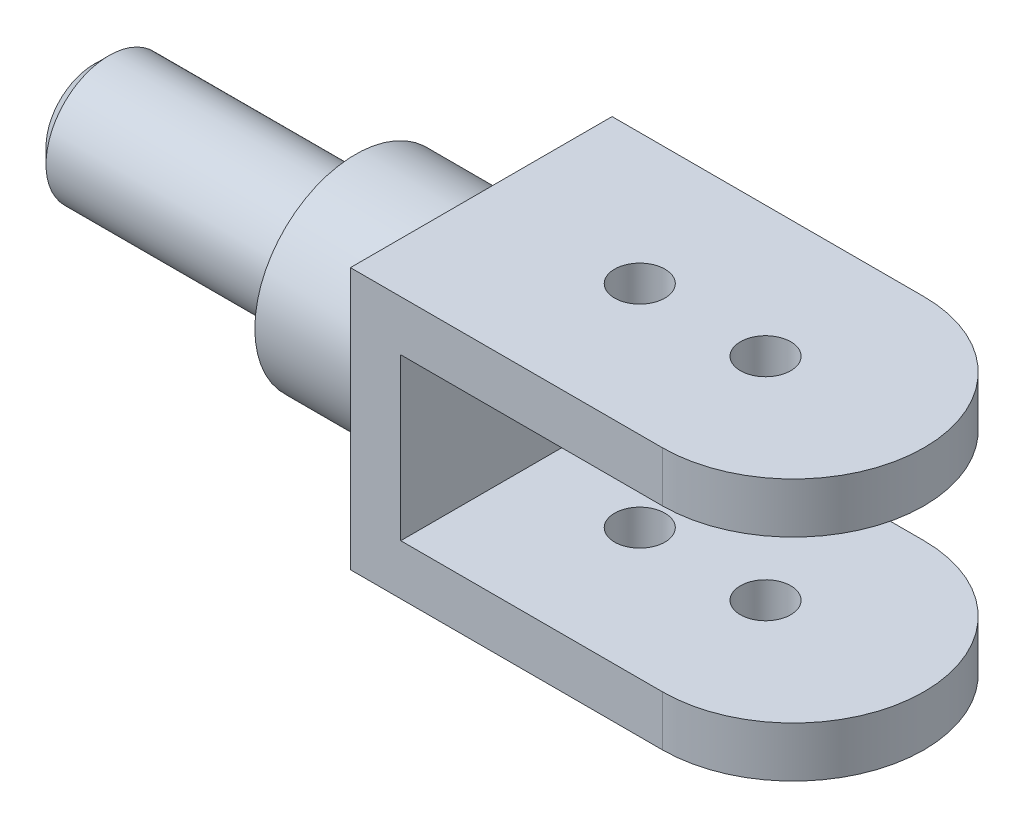
ISO-10303-21;
HEADER;
FILE_DESCRIPTION(('STEP AP214'),'2;1');
FILE_NAME('part.step','',(''),(''),'','','');
FILE_SCHEMA(('AUTOMOTIVE_DESIGN { 1 0 10303 214 1 1 1 1 }'));
ENDSEC;
DATA;
#1=APPLICATION_CONTEXT('core data for automotive mechanical design processes');
#2=APPLICATION_PROTOCOL_DEFINITION('international standard','automotive_design',2000,#1);
#3=PRODUCT_CONTEXT('',#1,'mechanical');
#4=PRODUCT('Part','Part','',(#3));
#5=PRODUCT_RELATED_PRODUCT_CATEGORY('part','',(#4));
#6=PRODUCT_DEFINITION_FORMATION('','',#4);
#7=PRODUCT_DEFINITION_CONTEXT('part definition',#1,'design');
#8=PRODUCT_DEFINITION('design','',#6,#7);
#9=PRODUCT_DEFINITION_SHAPE('','',#8);
#10=(LENGTH_UNIT() NAMED_UNIT(*) SI_UNIT(.MILLI.,.METRE.));
#11=(NAMED_UNIT(*) PLANE_ANGLE_UNIT() SI_UNIT($,.RADIAN.));
#12=(NAMED_UNIT(*) SI_UNIT($,.STERADIAN.) SOLID_ANGLE_UNIT());
#13=UNCERTAINTY_MEASURE_WITH_UNIT(LENGTH_MEASURE(1.E-05),#10,'distance_accuracy_value','');
#14=(GEOMETRIC_REPRESENTATION_CONTEXT(3) GLOBAL_UNCERTAINTY_ASSIGNED_CONTEXT((#13)) GLOBAL_UNIT_ASSIGNED_CONTEXT((#10,
#11,#12)) REPRESENTATION_CONTEXT('',''));
#15=CARTESIAN_POINT('',(0.,0.,0.));
#16=DIRECTION('',(0.,0.,1.));
#17=DIRECTION('',(1.,0.,0.));
#18=AXIS2_PLACEMENT_3D('',#15,#16,#17);
#19=CARTESIAN_POINT('',(0.,-52.,52.));
#20=DIRECTION('',(1.,0.,0.));
#21=DIRECTION('',(0.,0.,-1.));
#22=AXIS2_PLACEMENT_3D('',#19,#20,#21);
#23=PLANE('',#22);
#24=CARTESIAN_POINT('',(0.,-26.,26.));
#25=DIRECTION('',(1.,0.,0.));
#26=DIRECTION('',(0.,0.,-1.));
#27=AXIS2_PLACEMENT_3D('',#24,#25,#26);
#28=CIRCLE('',#27,23.);
#29=CARTESIAN_POINT('',(0.,-26.,3.00000000000002));
#30=VERTEX_POINT('',#29);
#31=EDGE_CURVE('E164',#30,#30,#28,.T.);
#32=ORIENTED_EDGE('',*,*,#31,.T.);
#33=EDGE_LOOP('',(#32));
#34=FACE_BOUND('',#33,.T.);
#35=DIRECTION('',(0.,-1.,0.));
#36=VECTOR('',#35,1.);
#37=CARTESIAN_POINT('',(0.,-52.,0.));
#38=LINE('',#37,#36);
#39=CARTESIAN_POINT('',(0.,0.,0.));
#40=VERTEX_POINT('',#39);
#41=CARTESIAN_POINT('',(0.,-52.,0.));
#42=VERTEX_POINT('',#41);
#43=EDGE_CURVE('E141',#40,#42,#38,.T.);
#44=ORIENTED_EDGE('',*,*,#43,.T.);
#45=DIRECTION('',(0.,0.,-1.));
#46=VECTOR('',#45,1.);
#47=CARTESIAN_POINT('',(0.,-52.,52.));
#48=LINE('',#47,#46);
#49=CARTESIAN_POINT('',(0.,-52.,52.));
#50=VERTEX_POINT('',#49);
#51=EDGE_CURVE('E159',#50,#42,#48,.T.);
#52=ORIENTED_EDGE('',*,*,#51,.F.);
#53=DIRECTION('',(0.,-1.,0.));
#54=VECTOR('',#53,1.);
#55=CARTESIAN_POINT('',(0.,-52.,52.));
#56=LINE('',#55,#54);
#57=CARTESIAN_POINT('',(0.,0.,52.));
#58=VERTEX_POINT('',#57);
#59=EDGE_CURVE('E146',#58,#50,#56,.T.);
#60=ORIENTED_EDGE('',*,*,#59,.F.);
#61=DIRECTION('',(0.,0.,-1.));
#62=VECTOR('',#61,1.);
#63=CARTESIAN_POINT('',(0.,0.,52.));
#64=LINE('',#63,#62);
#65=EDGE_CURVE('E153',#58,#40,#64,.T.);
#66=ORIENTED_EDGE('',*,*,#65,.T.);
#67=EDGE_LOOP('',(#44,#52,#60,#66));
#68=FACE_BOUND('',#67,.T.);
#69=ADVANCED_FACE('F50',(#34,#68),#23,.F.);
#70=CARTESIAN_POINT('',(88.,-52.,52.));
#71=DIRECTION('',(0.,1.,0.));
#72=DIRECTION('',(0.,0.,1.));
#73=AXIS2_PLACEMENT_3D('',#70,#71,#72);
#74=PLANE('',#73);
#75=CARTESIAN_POINT('',(31.5,-52.,26.));
#76=DIRECTION('',(0.,-1.,0.));
#77=DIRECTION('',(0.,0.,-1.));
#78=AXIS2_PLACEMENT_3D('',#75,#76,#77);
#79=CIRCLE('',#78,5.);
#80=CARTESIAN_POINT('',(31.5,-52.,21.));
#81=VERTEX_POINT('',#80);
#82=EDGE_CURVE('E512',#81,#81,#79,.T.);
#83=ORIENTED_EDGE('',*,*,#82,.F.);
#84=EDGE_LOOP('',(#83));
#85=FACE_BOUND('',#84,.T.);
#86=CARTESIAN_POINT('',(56.5,-52.,26.));
#87=DIRECTION('',(0.,-1.,0.));
#88=DIRECTION('',(0.,0.,-1.));
#89=AXIS2_PLACEMENT_3D('',#86,#87,#88);
#90=CIRCLE('',#89,5.);
#91=CARTESIAN_POINT('',(56.5,-52.,21.));
#92=VERTEX_POINT('',#91);
#93=EDGE_CURVE('E504',#92,#92,#90,.T.);
#94=ORIENTED_EDGE('',*,*,#93,.F.);
#95=EDGE_LOOP('',(#94));
#96=FACE_BOUND('',#95,.T.);
#97=DIRECTION('',(1.,0.,0.));
#98=VECTOR('',#97,1.);
#99=CARTESIAN_POINT('',(88.,-52.,0.));
#100=LINE('',#99,#98);
#101=CARTESIAN_POINT('',(62.,-52.,0.));
#102=VERTEX_POINT('',#101);
#103=EDGE_CURVE('E201',#42,#102,#100,.T.);
#104=ORIENTED_EDGE('',*,*,#103,.T.);
#105=CARTESIAN_POINT('',(62.,-52.,26.));
#106=DIRECTION('',(0.,-1.,0.));
#107=DIRECTION('',(0.,0.,-1.));
#108=AXIS2_PLACEMENT_3D('',#105,#106,#107);
#109=CIRCLE('',#108,26.);
#110=CARTESIAN_POINT('',(62.,-52.,52.));
#111=VERTEX_POINT('',#110);
#112=EDGE_CURVE('E131',#102,#111,#109,.T.);
#113=ORIENTED_EDGE('',*,*,#112,.T.);
#114=DIRECTION('',(1.,0.,0.));
#115=VECTOR('',#114,1.);
#116=CARTESIAN_POINT('',(88.,-52.,52.));
#117=LINE('',#116,#115);
#118=EDGE_CURVE('E100',#50,#111,#117,.T.);
#119=ORIENTED_EDGE('',*,*,#118,.F.);
#120=ORIENTED_EDGE('',*,*,#51,.T.);
#121=EDGE_LOOP('',(#104,#113,#119,#120));
#122=FACE_BOUND('',#121,.T.);
#123=ADVANCED_FACE('F213',(#85,#96,#122),#74,.F.);
#124=CARTESIAN_POINT('',(9.99999999999999,-42.,52.));
#125=DIRECTION('',(0.,-1.,0.));
#126=DIRECTION('',(0.,0.,-1.));
#127=AXIS2_PLACEMENT_3D('',#124,#125,#126);
#128=PLANE('',#127);
#129=CARTESIAN_POINT('',(31.5,-42.,26.));
#130=DIRECTION('',(0.,-1.,0.));
#131=DIRECTION('',(0.,0.,-1.));
#132=AXIS2_PLACEMENT_3D('',#129,#130,#131);
#133=CIRCLE('',#132,5.);
#134=CARTESIAN_POINT('',(31.5,-42.,21.));
#135=VERTEX_POINT('',#134);
#136=EDGE_CURVE('E180',#135,#135,#133,.T.);
#137=ORIENTED_EDGE('',*,*,#136,.T.);
#138=EDGE_LOOP('',(#137));
#139=FACE_BOUND('',#138,.T.);
#140=CARTESIAN_POINT('',(56.5,-42.,26.));
#141=DIRECTION('',(0.,-1.,0.));
#142=DIRECTION('',(0.,0.,-1.));
#143=AXIS2_PLACEMENT_3D('',#140,#141,#142);
#144=CIRCLE('',#143,5.);
#145=CARTESIAN_POINT('',(56.5,-42.,21.));
#146=VERTEX_POINT('',#145);
#147=EDGE_CURVE('E492',#146,#146,#144,.T.);
#148=ORIENTED_EDGE('',*,*,#147,.T.);
#149=EDGE_LOOP('',(#148));
#150=FACE_BOUND('',#149,.T.);
#151=DIRECTION('',(-1.,0.,0.));
#152=VECTOR('',#151,1.);
#153=CARTESIAN_POINT('',(9.99999999999999,-42.,52.));
#154=LINE('',#153,#152);
#155=CARTESIAN_POINT('',(62.,-42.,52.));
#156=VERTEX_POINT('',#155);
#157=CARTESIAN_POINT('',(9.99999999999999,-42.,52.));
#158=VERTEX_POINT('',#157);
#159=EDGE_CURVE('E195',#156,#158,#154,.T.);
#160=ORIENTED_EDGE('',*,*,#159,.F.);
#161=CARTESIAN_POINT('',(62.,-42.,26.));
#162=DIRECTION('',(0.,-1.,0.));
#163=DIRECTION('',(0.,0.,-1.));
#164=AXIS2_PLACEMENT_3D('',#161,#162,#163);
#165=CIRCLE('',#164,26.);
#166=CARTESIAN_POINT('',(62.,-42.,0.));
#167=VERTEX_POINT('',#166);
#168=EDGE_CURVE('E182',#167,#156,#165,.T.);
#169=ORIENTED_EDGE('',*,*,#168,.F.);
#170=DIRECTION('',(-1.,0.,0.));
#171=VECTOR('',#170,1.);
#172=CARTESIAN_POINT('',(9.99999999999999,-42.,0.));
#173=LINE('',#172,#171);
#174=CARTESIAN_POINT('',(9.99999999999999,-42.,0.));
#175=VERTEX_POINT('',#174);
#176=EDGE_CURVE('E152',#167,#175,#173,.T.);
#177=ORIENTED_EDGE('',*,*,#176,.T.);
#178=DIRECTION('',(0.,0.,-1.));
#179=VECTOR('',#178,1.);
#180=CARTESIAN_POINT('',(9.99999999999999,-42.,52.));
#181=LINE('',#180,#179);
#182=EDGE_CURVE('E157',#158,#175,#181,.T.);
#183=ORIENTED_EDGE('',*,*,#182,.F.);
#184=EDGE_LOOP('',(#160,#169,#177,#183));
#185=FACE_BOUND('',#184,.T.);
#186=ADVANCED_FACE('F207',(#139,#150,#185),#128,.F.);
#187=CARTESIAN_POINT('',(9.99999999999999,-10.,52.));
#188=DIRECTION('',(-1.,0.,0.));
#189=DIRECTION('',(0.,0.,1.));
#190=AXIS2_PLACEMENT_3D('',#187,#188,#189);
#191=PLANE('',#190);
#192=DIRECTION('',(0.,1.,0.));
#193=VECTOR('',#192,1.);
#194=CARTESIAN_POINT('',(9.99999999999999,-10.,0.));
#195=LINE('',#194,#193);
#196=CARTESIAN_POINT('',(9.99999999999999,-10.,0.));
#197=VERTEX_POINT('',#196);
#198=EDGE_CURVE('E81',#175,#197,#195,.T.);
#199=ORIENTED_EDGE('',*,*,#198,.T.);
#200=DIRECTION('',(0.,0.,-1.));
#201=VECTOR('',#200,1.);
#202=CARTESIAN_POINT('',(9.99999999999999,-10.,52.));
#203=LINE('',#202,#201);
#204=CARTESIAN_POINT('',(9.99999999999999,-10.,52.));
#205=VERTEX_POINT('',#204);
#206=EDGE_CURVE('E150',#205,#197,#203,.T.);
#207=ORIENTED_EDGE('',*,*,#206,.F.);
#208=DIRECTION('',(0.,1.,0.));
#209=VECTOR('',#208,1.);
#210=CARTESIAN_POINT('',(9.99999999999999,-10.,52.));
#211=LINE('',#210,#209);
#212=EDGE_CURVE('E191',#158,#205,#211,.T.);
#213=ORIENTED_EDGE('',*,*,#212,.F.);
#214=ORIENTED_EDGE('',*,*,#182,.T.);
#215=EDGE_LOOP('',(#199,#207,#213,#214));
#216=FACE_BOUND('',#215,.T.);
#217=ADVANCED_FACE('F209',(#216),#191,.F.);
#218=CARTESIAN_POINT('',(88.,-10.,52.));
#219=DIRECTION('',(0.,1.,0.));
#220=DIRECTION('',(0.,0.,1.));
#221=AXIS2_PLACEMENT_3D('',#218,#219,#220);
#222=PLANE('',#221);
#223=CARTESIAN_POINT('',(31.5,-10.,26.));
#224=DIRECTION('',(0.,1.,0.));
#225=DIRECTION('',(0.,0.,1.));
#226=AXIS2_PLACEMENT_3D('',#223,#224,#225);
#227=CIRCLE('',#226,5.);
#228=CARTESIAN_POINT('',(31.5,-10.,21.));
#229=VERTEX_POINT('',#228);
#230=EDGE_CURVE('E500',#229,#229,#227,.T.);
#231=ORIENTED_EDGE('',*,*,#230,.T.);
#232=EDGE_LOOP('',(#231));
#233=FACE_BOUND('',#232,.T.);
#234=CARTESIAN_POINT('',(56.5,-10.,26.));
#235=DIRECTION('',(0.,1.,0.));
#236=DIRECTION('',(0.,0.,1.));
#237=AXIS2_PLACEMENT_3D('',#234,#235,#236);
#238=CIRCLE('',#237,5.);
#239=CARTESIAN_POINT('',(56.5,-10.,21.));
#240=VERTEX_POINT('',#239);
#241=EDGE_CURVE('E498',#240,#240,#238,.T.);
#242=ORIENTED_EDGE('',*,*,#241,.T.);
#243=EDGE_LOOP('',(#242));
#244=FACE_BOUND('',#243,.T.);
#245=DIRECTION('',(1.,0.,0.));
#246=VECTOR('',#245,1.);
#247=CARTESIAN_POINT('',(88.,-10.,0.));
#248=LINE('',#247,#246);
#249=CARTESIAN_POINT('',(62.,-10.,0.));
#250=VERTEX_POINT('',#249);
#251=EDGE_CURVE('E142',#197,#250,#248,.T.);
#252=ORIENTED_EDGE('',*,*,#251,.T.);
#253=CARTESIAN_POINT('',(62.,-10.,26.));
#254=DIRECTION('',(0.,1.,0.));
#255=DIRECTION('',(0.,0.,1.));
#256=AXIS2_PLACEMENT_3D('',#253,#254,#255);
#257=CIRCLE('',#256,26.);
#258=CARTESIAN_POINT('',(62.,-10.,52.));
#259=VERTEX_POINT('',#258);
#260=EDGE_CURVE('E123',#259,#250,#257,.T.);
#261=ORIENTED_EDGE('',*,*,#260,.F.);
#262=DIRECTION('',(1.,0.,0.));
#263=VECTOR('',#262,1.);
#264=CARTESIAN_POINT('',(88.,-10.,52.));
#265=LINE('',#264,#263);
#266=EDGE_CURVE('E197',#205,#259,#265,.T.);
#267=ORIENTED_EDGE('',*,*,#266,.F.);
#268=ORIENTED_EDGE('',*,*,#206,.T.);
#269=EDGE_LOOP('',(#252,#261,#267,#268));
#270=FACE_BOUND('',#269,.T.);
#271=ADVANCED_FACE('F147',(#233,#244,#270),#222,.F.);
#272=CARTESIAN_POINT('',(0.,0.,52.));
#273=DIRECTION('',(0.,-1.,0.));
#274=DIRECTION('',(0.,0.,-1.));
#275=AXIS2_PLACEMENT_3D('',#272,#273,#274);
#276=PLANE('',#275);
#277=CARTESIAN_POINT('',(31.5,0.,26.));
#278=DIRECTION('',(0.,-1.,0.));
#279=DIRECTION('',(0.,0.,-1.));
#280=AXIS2_PLACEMENT_3D('',#277,#278,#279);
#281=CIRCLE('',#280,5.);
#282=CARTESIAN_POINT('',(31.5,0.,21.));
#283=VERTEX_POINT('',#282);
#284=EDGE_CURVE('E505',#283,#283,#281,.T.);
#285=ORIENTED_EDGE('',*,*,#284,.T.);
#286=EDGE_LOOP('',(#285));
#287=FACE_BOUND('',#286,.T.);
#288=CARTESIAN_POINT('',(56.5,0.,26.));
#289=DIRECTION('',(0.,-1.,0.));
#290=DIRECTION('',(0.,0.,-1.));
#291=AXIS2_PLACEMENT_3D('',#288,#289,#290);
#292=CIRCLE('',#291,5.);
#293=CARTESIAN_POINT('',(56.5,0.,21.));
#294=VERTEX_POINT('',#293);
#295=EDGE_CURVE('E507',#294,#294,#292,.T.);
#296=ORIENTED_EDGE('',*,*,#295,.T.);
#297=EDGE_LOOP('',(#296));
#298=FACE_BOUND('',#297,.T.);
#299=DIRECTION('',(-1.,0.,0.));
#300=VECTOR('',#299,1.);
#301=CARTESIAN_POINT('',(0.,0.,52.));
#302=LINE('',#301,#300);
#303=CARTESIAN_POINT('',(62.,0.,52.));
#304=VERTEX_POINT('',#303);
#305=EDGE_CURVE('E63',#304,#58,#302,.T.);
#306=ORIENTED_EDGE('',*,*,#305,.F.);
#307=CARTESIAN_POINT('',(62.,0.,26.));
#308=DIRECTION('',(0.,1.,0.));
#309=DIRECTION('',(0.,0.,1.));
#310=AXIS2_PLACEMENT_3D('',#307,#308,#309);
#311=CIRCLE('',#310,26.);
#312=CARTESIAN_POINT('',(62.,0.,0.));
#313=VERTEX_POINT('',#312);
#314=EDGE_CURVE('E133',#304,#313,#311,.T.);
#315=ORIENTED_EDGE('',*,*,#314,.T.);
#316=DIRECTION('',(-1.,0.,0.));
#317=VECTOR('',#316,1.);
#318=CARTESIAN_POINT('',(0.,0.,0.));
#319=LINE('',#318,#317);
#320=EDGE_CURVE('E91',#313,#40,#319,.T.);
#321=ORIENTED_EDGE('',*,*,#320,.T.);
#322=ORIENTED_EDGE('',*,*,#65,.F.);
#323=EDGE_LOOP('',(#306,#315,#321,#322));
#324=FACE_BOUND('',#323,.T.);
#325=ADVANCED_FACE('F220',(#287,#298,#324),#276,.F.);
#326=CARTESIAN_POINT('',(0.,0.,52.));
#327=DIRECTION('',(0.,0.,-1.));
#328=DIRECTION('',(-1.,0.,0.));
#329=AXIS2_PLACEMENT_3D('',#326,#327,#328);
#330=PLANE('',#329);
#331=ORIENTED_EDGE('',*,*,#118,.T.);
#332=DIRECTION('',(0.,-1.,0.));
#333=VECTOR('',#332,1.);
#334=CARTESIAN_POINT('',(62.,18.,52.));
#335=LINE('',#334,#333);
#336=EDGE_CURVE('E187',#156,#111,#335,.T.);
#337=ORIENTED_EDGE('',*,*,#336,.F.);
#338=ORIENTED_EDGE('',*,*,#159,.T.);
#339=ORIENTED_EDGE('',*,*,#212,.T.);
#340=ORIENTED_EDGE('',*,*,#266,.T.);
#341=EDGE_CURVE('E126',#304,#259,#335,.T.);
#342=ORIENTED_EDGE('',*,*,#341,.F.);
#343=ORIENTED_EDGE('',*,*,#305,.T.);
#344=ORIENTED_EDGE('',*,*,#59,.T.);
#345=EDGE_LOOP('',(#331,#337,#338,#339,#340,#342,#343,#344));
#346=FACE_BOUND('',#345,.T.);
#347=ADVANCED_FACE('F208',(#346),#330,.F.);
#348=CARTESIAN_POINT('',(0.,0.,0.));
#349=DIRECTION('',(0.,0.,-1.));
#350=DIRECTION('',(-1.,0.,0.));
#351=AXIS2_PLACEMENT_3D('',#348,#349,#350);
#352=PLANE('',#351);
#353=DIRECTION('',(0.,-1.,0.));
#354=VECTOR('',#353,1.);
#355=CARTESIAN_POINT('',(62.,18.,0.));
#356=LINE('',#355,#354);
#357=EDGE_CURVE('E144',#167,#102,#356,.T.);
#358=ORIENTED_EDGE('',*,*,#357,.T.);
#359=ORIENTED_EDGE('',*,*,#103,.F.);
#360=ORIENTED_EDGE('',*,*,#43,.F.);
#361=ORIENTED_EDGE('',*,*,#320,.F.);
#362=EDGE_CURVE('E129',#313,#250,#356,.T.);
#363=ORIENTED_EDGE('',*,*,#362,.T.);
#364=ORIENTED_EDGE('',*,*,#251,.F.);
#365=ORIENTED_EDGE('',*,*,#198,.F.);
#366=ORIENTED_EDGE('',*,*,#176,.F.);
#367=EDGE_LOOP('',(#358,#359,#360,#361,#363,#364,#365,#366));
#368=FACE_BOUND('',#367,.T.);
#369=ADVANCED_FACE('F139',(#368),#352,.T.);
#370=CARTESIAN_POINT('',(62.,-42.,26.));
#371=DIRECTION('',(0.,-1.,0.));
#372=DIRECTION('',(0.,0.,-1.));
#373=AXIS2_PLACEMENT_3D('',#370,#371,#372);
#374=CYLINDRICAL_SURFACE('',#373,26.);
#375=ORIENTED_EDGE('',*,*,#112,.F.);
#376=ORIENTED_EDGE('',*,*,#357,.F.);
#377=ORIENTED_EDGE('',*,*,#168,.T.);
#378=ORIENTED_EDGE('',*,*,#336,.T.);
#379=EDGE_LOOP('',(#375,#376,#377,#378));
#380=FACE_BOUND('',#379,.T.);
#381=ADVANCED_FACE('F214',(#380),#374,.T.);
#382=CARTESIAN_POINT('',(62.,-10.,26.));
#383=DIRECTION('',(0.,1.,0.));
#384=DIRECTION('',(0.,0.,1.));
#385=AXIS2_PLACEMENT_3D('',#382,#383,#384);
#386=CYLINDRICAL_SURFACE('',#385,26.);
#387=ORIENTED_EDGE('',*,*,#314,.F.);
#388=ORIENTED_EDGE('',*,*,#341,.T.);
#389=ORIENTED_EDGE('',*,*,#260,.T.);
#390=ORIENTED_EDGE('',*,*,#362,.F.);
#391=EDGE_LOOP('',(#387,#388,#389,#390));
#392=FACE_BOUND('',#391,.T.);
#393=ADVANCED_FACE('F130',(#392),#386,.T.);
#394=CARTESIAN_POINT('',(-25.,-26.,26.));
#395=DIRECTION('',(1.,0.,0.));
#396=DIRECTION('',(0.,0.,-1.));
#397=AXIS2_PLACEMENT_3D('',#394,#395,#396);
#398=CYLINDRICAL_SURFACE('',#397,20.);
#399=CARTESIAN_POINT('',(-3.00000000000002,-26.,26.));
#400=DIRECTION('',(1.,0.,0.));
#401=DIRECTION('',(0.,0.,-1.));
#402=AXIS2_PLACEMENT_3D('',#399,#400,#401);
#403=CIRCLE('',#402,20.);
#404=CARTESIAN_POINT('',(-3.00000000000002,-26.,6.));
#405=VERTEX_POINT('',#404);
#406=EDGE_CURVE('E162',#405,#405,#403,.F.);
#407=ORIENTED_EDGE('',*,*,#406,.T.);
#408=EDGE_LOOP('',(#407));
#409=FACE_BOUND('',#408,.T.);
#410=CARTESIAN_POINT('',(-25.,-26.,26.));
#411=DIRECTION('',(-1.,0.,0.));
#412=DIRECTION('',(0.,0.,1.));
#413=AXIS2_PLACEMENT_3D('',#410,#411,#412);
#414=CIRCLE('',#413,20.);
#415=CARTESIAN_POINT('',(-25.,-26.,46.));
#416=VERTEX_POINT('',#415);
#417=EDGE_CURVE('E177',#416,#416,#414,.T.);
#418=ORIENTED_EDGE('',*,*,#417,.F.);
#419=EDGE_LOOP('',(#418));
#420=FACE_BOUND('',#419,.T.);
#421=ADVANCED_FACE('F258',(#409,#420),#398,.T.);
#422=CARTESIAN_POINT('',(-25.,-26.,26.));
#423=DIRECTION('',(-1.,0.,0.));
#424=DIRECTION('',(0.,0.,1.));
#425=AXIS2_PLACEMENT_3D('',#422,#423,#424);
#426=PLANE('',#425);
#427=CARTESIAN_POINT('',(-25.,-26.,26.));
#428=DIRECTION('',(-1.,0.,0.));
#429=DIRECTION('',(0.,0.,1.));
#430=AXIS2_PLACEMENT_3D('',#427,#428,#429);
#431=CIRCLE('',#430,12.5);
#432=CARTESIAN_POINT('',(-25.,-26.,13.5));
#433=VERTEX_POINT('',#432);
#434=EDGE_CURVE('E170',#433,#433,#431,.T.);
#435=ORIENTED_EDGE('',*,*,#434,.F.);
#436=EDGE_LOOP('',(#435));
#437=FACE_BOUND('',#436,.T.);
#438=ORIENTED_EDGE('',*,*,#417,.T.);
#439=EDGE_LOOP('',(#438));
#440=FACE_BOUND('',#439,.T.);
#441=ADVANCED_FACE('F249',(#437,#440),#426,.T.);
#442=CARTESIAN_POINT('',(-3.00000000000002,-26.,26.));
#443=DIRECTION('',(1.,0.,0.));
#444=DIRECTION('',(0.,0.,-1.));
#445=AXIS2_PLACEMENT_3D('',#442,#443,#444);
#446=CONICAL_SURFACE('',#445,20.,0.785398163397443);
#447=ORIENTED_EDGE('',*,*,#31,.F.);
#448=EDGE_LOOP('',(#447));
#449=FACE_BOUND('',#448,.T.);
#450=ORIENTED_EDGE('',*,*,#406,.F.);
#451=EDGE_LOOP('',(#450));
#452=FACE_BOUND('',#451,.T.);
#453=ADVANCED_FACE('F244',(#449,#452),#446,.T.);
#454=CARTESIAN_POINT('',(-77.,-26.,26.));
#455=DIRECTION('',(1.,0.,0.));
#456=DIRECTION('',(0.,0.,-1.));
#457=AXIS2_PLACEMENT_3D('',#454,#455,#456);
#458=CYLINDRICAL_SURFACE('',#457,12.5);
#459=CARTESIAN_POINT('',(-74.0000000000001,-26.,26.));
#460=DIRECTION('',(-1.,0.,0.));
#461=DIRECTION('',(0.,0.,1.));
#462=AXIS2_PLACEMENT_3D('',#459,#460,#461);
#463=CIRCLE('',#462,12.5);
#464=CARTESIAN_POINT('',(-74.0000000000001,-26.,13.5));
#465=VERTEX_POINT('',#464);
#466=EDGE_CURVE('E11',#465,#465,#463,.F.);
#467=CARTESIAN_POINT('',(-74.0000000000001,-26.,13.5));
#468=CARTESIAN_POINT('',(-73.4895833333334,-26.,13.5));
#469=CARTESIAN_POINT('',(-72.9791666666668,-26.,13.5));
#470=CARTESIAN_POINT('',(-71.9583333333334,-26.,13.5));
#471=CARTESIAN_POINT('',(-71.4479166666668,-26.,13.5));
#472=CARTESIAN_POINT('',(-70.4270833333334,-26.,13.5));
#473=CARTESIAN_POINT('',(-69.9166666666668,-26.,13.5));
#474=CARTESIAN_POINT('',(-68.8958333333334,-26.,13.5));
#475=CARTESIAN_POINT('',(-68.3854166666668,-26.,13.5));
#476=CARTESIAN_POINT('',(-67.3645833333334,-26.,13.5));
#477=CARTESIAN_POINT('',(-66.8541666666668,-26.,13.5));
#478=CARTESIAN_POINT('',(-65.8333333333334,-26.,13.5));
#479=CARTESIAN_POINT('',(-65.3229166666668,-26.,13.5));
#480=CARTESIAN_POINT('',(-64.3020833333334,-26.,13.5));
#481=CARTESIAN_POINT('',(-63.7916666666668,-26.,13.5));
#482=CARTESIAN_POINT('',(-62.7708333333334,-26.,13.5));
#483=CARTESIAN_POINT('',(-62.2604166666668,-26.,13.5));
#484=CARTESIAN_POINT('',(-61.2395833333334,-26.,13.5));
#485=CARTESIAN_POINT('',(-60.7291666666667,-26.,13.5));
#486=CARTESIAN_POINT('',(-59.7083333333334,-26.,13.5));
#487=CARTESIAN_POINT('',(-59.1979166666667,-26.,13.5));
#488=CARTESIAN_POINT('',(-58.1770833333334,-26.,13.5));
#489=CARTESIAN_POINT('',(-57.6666666666667,-26.,13.5));
#490=CARTESIAN_POINT('',(-56.6458333333334,-26.,13.5));
#491=CARTESIAN_POINT('',(-56.1354166666667,-26.,13.5));
#492=CARTESIAN_POINT('',(-55.1145833333334,-26.,13.5));
#493=CARTESIAN_POINT('',(-54.6041666666667,-26.,13.5));
#494=CARTESIAN_POINT('',(-53.5833333333334,-26.,13.5));
#495=CARTESIAN_POINT('',(-53.0729166666667,-26.,13.5));
#496=CARTESIAN_POINT('',(-52.0520833333334,-26.,13.5));
#497=CARTESIAN_POINT('',(-51.5416666666667,-26.,13.5));
#498=CARTESIAN_POINT('',(-50.5208333333334,-26.,13.5));
#499=CARTESIAN_POINT('',(-50.0104166666667,-26.,13.5));
#500=CARTESIAN_POINT('',(-48.9895833333334,-26.,13.5));
#501=CARTESIAN_POINT('',(-48.4791666666667,-26.,13.5));
#502=CARTESIAN_POINT('',(-47.4583333333334,-26.,13.5));
#503=CARTESIAN_POINT('',(-46.9479166666667,-26.,13.5));
#504=CARTESIAN_POINT('',(-45.9270833333334,-26.,13.5));
#505=CARTESIAN_POINT('',(-45.4166666666667,-26.,13.5));
#506=CARTESIAN_POINT('',(-44.3958333333334,-26.,13.5));
#507=CARTESIAN_POINT('',(-43.8854166666667,-26.,13.5));
#508=CARTESIAN_POINT('',(-42.8645833333334,-26.,13.5));
#509=CARTESIAN_POINT('',(-42.3541666666667,-26.,13.5));
#510=CARTESIAN_POINT('',(-41.3333333333334,-26.,13.5));
#511=CARTESIAN_POINT('',(-40.8229166666667,-26.,13.5));
#512=CARTESIAN_POINT('',(-39.8020833333334,-26.,13.5));
#513=CARTESIAN_POINT('',(-39.2916666666667,-26.,13.5));
#514=CARTESIAN_POINT('',(-38.2708333333334,-26.,13.5));
#515=CARTESIAN_POINT('',(-37.7604166666667,-26.,13.5));
#516=CARTESIAN_POINT('',(-36.7395833333334,-26.,13.5));
#517=CARTESIAN_POINT('',(-36.2291666666667,-26.,13.5));
#518=CARTESIAN_POINT('',(-35.2083333333334,-26.,13.5));
#519=CARTESIAN_POINT('',(-34.6979166666667,-26.,13.5));
#520=CARTESIAN_POINT('',(-33.6770833333334,-26.,13.5));
#521=CARTESIAN_POINT('',(-33.1666666666667,-26.,13.5));
#522=CARTESIAN_POINT('',(-32.1458333333333,-26.,13.5));
#523=CARTESIAN_POINT('',(-31.6354166666667,-26.,13.5));
#524=CARTESIAN_POINT('',(-30.6145833333333,-26.,13.5));
#525=CARTESIAN_POINT('',(-30.1041666666667,-26.,13.5));
#526=CARTESIAN_POINT('',(-29.0833333333333,-26.,13.5));
#527=CARTESIAN_POINT('',(-28.5729166666667,-26.,13.5));
#528=CARTESIAN_POINT('',(-27.5520833333333,-26.,13.5));
#529=CARTESIAN_POINT('',(-27.0416666666667,-26.,13.5));
#530=CARTESIAN_POINT('',(-26.0208333333333,-26.,13.5));
#531=CARTESIAN_POINT('',(-25.5104166666667,-26.,13.5));
#532=CARTESIAN_POINT('',(-25.,-26.,13.5));
#533=B_SPLINE_CURVE_WITH_KNOTS('',3,(#467,#468,#469,#470,#471,#472,#473,#474,#475,#476,#477,
#478,#479,#480,#481,#482,#483,#484,#485,#486,#487,#488,#489,#490,#491,#492,#493,#494,#495,#496,
#497,#498,#499,#500,#501,#502,#503,#504,#505,#506,#507,#508,#509,#510,#511,#512,#513,#514,#515,
#516,#517,#518,#519,#520,#521,#522,#523,#524,#525,#526,#527,#528,#529,#530,#531,#532),
.UNSPECIFIED.,.F.,.F.,(4,2,2,2,2,2,2,2,2,2,2,2,2,2,2,2,2,2,2,2,2,2,2,2,2,2,2,2,2,2,2,2,4),(0.,
1.53125,3.0625,4.59375000000001,6.12500000000001,7.65625000000002,9.18750000000001,10.71875,
12.25,13.78125,15.3125,16.84375,18.375,19.90625,21.4375,22.96875,24.5,26.0312500000001,
27.5625000000001,29.0937500000001,30.6250000000001,32.1562500000001,33.6875000000001,
35.2187500000001,36.7500000000001,38.2812500000001,39.8125000000001,41.3437500000001,
42.8750000000001,44.4062500000001,45.9375000000001,47.4687500000001,49.0000000000001),.UNSPECIFIED.);
#534=EDGE_CURVE('BSEAM248',#465,#433,#533,.T.);
#535=ORIENTED_EDGE('',*,*,#466,.T.);
#536=ORIENTED_EDGE('',*,*,#434,.T.);
#537=ORIENTED_EDGE('',*,*,#534,.T.);
#538=ORIENTED_EDGE('',*,*,#534,.F.);
#539=EDGE_LOOP('',(#535,#537,#536,#538));
#540=FACE_BOUND('',#539,.T.);
#541=ADVANCED_FACE('F248',(#540),#458,.T.);
#542=CARTESIAN_POINT('',(-77.,-26.,26.));
#543=DIRECTION('',(-1.,0.,0.));
#544=DIRECTION('',(0.,0.,1.));
#545=AXIS2_PLACEMENT_3D('',#542,#543,#544);
#546=PLANE('',#545);
#547=CARTESIAN_POINT('',(-77.,-26.,26.));
#548=DIRECTION('',(-1.,0.,0.));
#549=DIRECTION('',(0.,0.,1.));
#550=AXIS2_PLACEMENT_3D('',#547,#548,#549);
#551=CIRCLE('',#550,9.50000000000012);
#552=CARTESIAN_POINT('',(-77.,-26.,35.5000000000001));
#553=VERTEX_POINT('',#552);
#554=EDGE_CURVE('E60',#553,#553,#551,.T.);
#555=ORIENTED_EDGE('',*,*,#554,.T.);
#556=EDGE_LOOP('',(#555));
#557=FACE_BOUND('',#556,.T.);
#558=ADVANCED_FACE('F257',(#557),#546,.T.);
#559=CARTESIAN_POINT('',(-77.,-26.,26.));
#560=DIRECTION('',(1.,0.,0.));
#561=DIRECTION('',(0.,0.,-1.));
#562=AXIS2_PLACEMENT_3D('',#559,#560,#561);
#563=CONICAL_SURFACE('',#562,9.50000000000012,0.785398163397449);
#564=ORIENTED_EDGE('',*,*,#466,.F.);
#565=EDGE_LOOP('',(#564));
#566=FACE_BOUND('',#565,.T.);
#567=ORIENTED_EDGE('',*,*,#554,.F.);
#568=EDGE_LOOP('',(#567));
#569=FACE_BOUND('',#568,.T.);
#570=ADVANCED_FACE('F49',(#566,#569),#563,.T.);
#571=CARTESIAN_POINT('',(56.5,0.,26.));
#572=DIRECTION('',(0.,-1.,0.));
#573=DIRECTION('',(0.,0.,-1.));
#574=AXIS2_PLACEMENT_3D('',#571,#572,#573);
#575=CYLINDRICAL_SURFACE('',#574,5.);
#576=CARTESIAN_POINT('',(56.5,0.,21.));
#577=CARTESIAN_POINT('',(56.5,-0.104166666666674,21.));
#578=CARTESIAN_POINT('',(56.5,-0.20833333333334,21.));
#579=CARTESIAN_POINT('',(56.5,-0.416666666666673,21.));
#580=CARTESIAN_POINT('',(56.5,-0.52083333333334,21.));
#581=CARTESIAN_POINT('',(56.5,-0.729166666666673,21.));
#582=CARTESIAN_POINT('',(56.5,-0.83333333333334,21.));
#583=CARTESIAN_POINT('',(56.5,-1.04166666666667,21.));
#584=CARTESIAN_POINT('',(56.5,-1.14583333333334,21.));
#585=CARTESIAN_POINT('',(56.5,-1.35416666666667,21.));
#586=CARTESIAN_POINT('',(56.5,-1.45833333333334,21.));
#587=CARTESIAN_POINT('',(56.5,-1.66666666666667,21.));
#588=CARTESIAN_POINT('',(56.5,-1.77083333333334,21.));
#589=CARTESIAN_POINT('',(56.5,-1.97916666666667,21.));
#590=CARTESIAN_POINT('',(56.5,-2.08333333333334,21.));
#591=CARTESIAN_POINT('',(56.5,-2.29166666666667,21.));
#592=CARTESIAN_POINT('',(56.5,-2.39583333333334,21.));
#593=CARTESIAN_POINT('',(56.5,-2.60416666666667,21.));
#594=CARTESIAN_POINT('',(56.5,-2.70833333333334,21.));
#595=CARTESIAN_POINT('',(56.5,-2.91666666666667,21.));
#596=CARTESIAN_POINT('',(56.5,-3.02083333333334,21.));
#597=CARTESIAN_POINT('',(56.5,-3.22916666666667,21.));
#598=CARTESIAN_POINT('',(56.5,-3.33333333333334,21.));
#599=CARTESIAN_POINT('',(56.5,-3.54166666666667,21.));
#600=CARTESIAN_POINT('',(56.5,-3.64583333333334,21.));
#601=CARTESIAN_POINT('',(56.5,-3.85416666666667,21.));
#602=CARTESIAN_POINT('',(56.5,-3.95833333333334,21.));
#603=CARTESIAN_POINT('',(56.5,-4.16666666666667,21.));
#604=CARTESIAN_POINT('',(56.5,-4.27083333333334,21.));
#605=CARTESIAN_POINT('',(56.5,-4.47916666666667,21.));
#606=CARTESIAN_POINT('',(56.5,-4.58333333333334,21.));
#607=CARTESIAN_POINT('',(56.5,-4.79166666666667,21.));
#608=CARTESIAN_POINT('',(56.5,-4.89583333333334,21.));
#609=CARTESIAN_POINT('',(56.5,-5.10416666666667,21.));
#610=CARTESIAN_POINT('',(56.5,-5.20833333333334,21.));
#611=CARTESIAN_POINT('',(56.5,-5.41666666666667,21.));
#612=CARTESIAN_POINT('',(56.5,-5.52083333333334,21.));
#613=CARTESIAN_POINT('',(56.5,-5.72916666666667,21.));
#614=CARTESIAN_POINT('',(56.5,-5.83333333333334,21.));
#615=CARTESIAN_POINT('',(56.5,-6.04166666666667,21.));
#616=CARTESIAN_POINT('',(56.5,-6.14583333333334,21.));
#617=CARTESIAN_POINT('',(56.5,-6.35416666666667,21.));
#618=CARTESIAN_POINT('',(56.5,-6.45833333333334,21.));
#619=CARTESIAN_POINT('',(56.5,-6.66666666666667,21.));
#620=CARTESIAN_POINT('',(56.5,-6.77083333333334,21.));
#621=CARTESIAN_POINT('',(56.5,-6.97916666666667,21.));
#622=CARTESIAN_POINT('',(56.5,-7.08333333333334,21.));
#623=CARTESIAN_POINT('',(56.5,-7.29166666666667,21.));
#624=CARTESIAN_POINT('',(56.5,-7.39583333333334,21.));
#625=CARTESIAN_POINT('',(56.5,-7.60416666666667,21.));
#626=CARTESIAN_POINT('',(56.5,-7.70833333333334,21.));
#627=CARTESIAN_POINT('',(56.5,-7.91666666666667,21.));
#628=CARTESIAN_POINT('',(56.5,-8.02083333333334,21.));
#629=CARTESIAN_POINT('',(56.5,-8.22916666666667,21.));
#630=CARTESIAN_POINT('',(56.5,-8.33333333333334,21.));
#631=CARTESIAN_POINT('',(56.5,-8.54166666666667,21.));
#632=CARTESIAN_POINT('',(56.5,-8.64583333333333,21.));
#633=CARTESIAN_POINT('',(56.5,-8.85416666666667,21.));
#634=CARTESIAN_POINT('',(56.5,-8.95833333333333,21.));
#635=CARTESIAN_POINT('',(56.5,-9.16666666666667,21.));
#636=CARTESIAN_POINT('',(56.5,-9.27083333333333,21.));
#637=CARTESIAN_POINT('',(56.5,-9.47916666666667,21.));
#638=CARTESIAN_POINT('',(56.5,-9.58333333333333,21.));
#639=CARTESIAN_POINT('',(56.5,-9.79166666666667,21.));
#640=CARTESIAN_POINT('',(56.5,-9.89583333333333,21.));
#641=CARTESIAN_POINT('',(56.5,-10.,21.));
#642=B_SPLINE_CURVE_WITH_KNOTS('',3,(#576,#577,#578,#579,#580,#581,#582,#583,#584,#585,#586,
#587,#588,#589,#590,#591,#592,#593,#594,#595,#596,#597,#598,#599,#600,#601,#602,#603,#604,#605,
#606,#607,#608,#609,#610,#611,#612,#613,#614,#615,#616,#617,#618,#619,#620,#621,#622,#623,#624,
#625,#626,#627,#628,#629,#630,#631,#632,#633,#634,#635,#636,#637,#638,#639,#640,#641),
.UNSPECIFIED.,.F.,.F.,(4,2,2,2,2,2,2,2,2,2,2,2,2,2,2,2,2,2,2,2,2,2,2,2,2,2,2,2,2,2,2,2,4),(0.,
0.3125,0.625,0.937499999999999,1.25,1.5625,1.875,2.1875,2.5,2.8125,3.125,3.4375,3.75,4.0625,
4.375,4.6875,5.,5.3125,5.625,5.9375,6.25,6.5625,6.875,7.18749999999999,7.5,7.8125,
8.12499999999999,8.43749999999999,8.74999999999999,9.06249999999999,9.37499999999999,
9.68749999999999,9.99999999999999),.UNSPECIFIED.);
#643=EDGE_CURVE('BSEAM312',#294,#240,#642,.T.);
#644=ORIENTED_EDGE('',*,*,#295,.F.);
#645=ORIENTED_EDGE('',*,*,#241,.F.);
#646=ORIENTED_EDGE('',*,*,#643,.T.);
#647=ORIENTED_EDGE('',*,*,#643,.F.);
#648=EDGE_LOOP('',(#644,#646,#645,#647));
#649=FACE_BOUND('',#648,.T.);
#650=ADVANCED_FACE('F312',(#649),#575,.F.);
#651=CARTESIAN_POINT('',(31.5,0.,26.));
#652=DIRECTION('',(0.,-1.,0.));
#653=DIRECTION('',(0.,0.,-1.));
#654=AXIS2_PLACEMENT_3D('',#651,#652,#653);
#655=CYLINDRICAL_SURFACE('',#654,5.);
#656=CARTESIAN_POINT('',(31.5,0.,21.));
#657=CARTESIAN_POINT('',(31.5,-0.104166666666674,21.));
#658=CARTESIAN_POINT('',(31.5,-0.20833333333334,21.));
#659=CARTESIAN_POINT('',(31.5,-0.416666666666673,21.));
#660=CARTESIAN_POINT('',(31.5,-0.52083333333334,21.));
#661=CARTESIAN_POINT('',(31.5,-0.729166666666673,21.));
#662=CARTESIAN_POINT('',(31.5,-0.83333333333334,21.));
#663=CARTESIAN_POINT('',(31.5,-1.04166666666667,21.));
#664=CARTESIAN_POINT('',(31.5,-1.14583333333334,21.));
#665=CARTESIAN_POINT('',(31.5,-1.35416666666667,21.));
#666=CARTESIAN_POINT('',(31.5,-1.45833333333334,21.));
#667=CARTESIAN_POINT('',(31.5,-1.66666666666667,21.));
#668=CARTESIAN_POINT('',(31.5,-1.77083333333334,21.));
#669=CARTESIAN_POINT('',(31.5,-1.97916666666667,21.));
#670=CARTESIAN_POINT('',(31.5,-2.08333333333334,21.));
#671=CARTESIAN_POINT('',(31.5,-2.29166666666667,21.));
#672=CARTESIAN_POINT('',(31.5,-2.39583333333334,21.));
#673=CARTESIAN_POINT('',(31.5,-2.60416666666667,21.));
#674=CARTESIAN_POINT('',(31.5,-2.70833333333334,21.));
#675=CARTESIAN_POINT('',(31.5,-2.91666666666667,21.));
#676=CARTESIAN_POINT('',(31.5,-3.02083333333334,21.));
#677=CARTESIAN_POINT('',(31.5,-3.22916666666667,21.));
#678=CARTESIAN_POINT('',(31.5,-3.33333333333334,21.));
#679=CARTESIAN_POINT('',(31.5,-3.54166666666667,21.));
#680=CARTESIAN_POINT('',(31.5,-3.64583333333334,21.));
#681=CARTESIAN_POINT('',(31.5,-3.85416666666667,21.));
#682=CARTESIAN_POINT('',(31.5,-3.95833333333334,21.));
#683=CARTESIAN_POINT('',(31.5,-4.16666666666667,21.));
#684=CARTESIAN_POINT('',(31.5,-4.27083333333334,21.));
#685=CARTESIAN_POINT('',(31.5,-4.47916666666667,21.));
#686=CARTESIAN_POINT('',(31.5,-4.58333333333334,21.));
#687=CARTESIAN_POINT('',(31.5,-4.79166666666667,21.));
#688=CARTESIAN_POINT('',(31.5,-4.89583333333334,21.));
#689=CARTESIAN_POINT('',(31.5,-5.10416666666667,21.));
#690=CARTESIAN_POINT('',(31.5,-5.20833333333334,21.));
#691=CARTESIAN_POINT('',(31.5,-5.41666666666667,21.));
#692=CARTESIAN_POINT('',(31.5,-5.52083333333334,21.));
#693=CARTESIAN_POINT('',(31.5,-5.72916666666667,21.));
#694=CARTESIAN_POINT('',(31.5,-5.83333333333334,21.));
#695=CARTESIAN_POINT('',(31.5,-6.04166666666667,21.));
#696=CARTESIAN_POINT('',(31.5,-6.14583333333334,21.));
#697=CARTESIAN_POINT('',(31.5,-6.35416666666667,21.));
#698=CARTESIAN_POINT('',(31.5,-6.45833333333334,21.));
#699=CARTESIAN_POINT('',(31.5,-6.66666666666667,21.));
#700=CARTESIAN_POINT('',(31.5,-6.77083333333334,21.));
#701=CARTESIAN_POINT('',(31.5,-6.97916666666667,21.));
#702=CARTESIAN_POINT('',(31.5,-7.08333333333334,21.));
#703=CARTESIAN_POINT('',(31.5,-7.29166666666667,21.));
#704=CARTESIAN_POINT('',(31.5,-7.39583333333334,21.));
#705=CARTESIAN_POINT('',(31.5,-7.60416666666667,21.));
#706=CARTESIAN_POINT('',(31.5,-7.70833333333334,21.));
#707=CARTESIAN_POINT('',(31.5,-7.91666666666667,21.));
#708=CARTESIAN_POINT('',(31.5,-8.02083333333334,21.));
#709=CARTESIAN_POINT('',(31.5,-8.22916666666667,21.));
#710=CARTESIAN_POINT('',(31.5,-8.33333333333334,21.));
#711=CARTESIAN_POINT('',(31.5,-8.54166666666667,21.));
#712=CARTESIAN_POINT('',(31.5,-8.64583333333333,21.));
#713=CARTESIAN_POINT('',(31.5,-8.85416666666667,21.));
#714=CARTESIAN_POINT('',(31.5,-8.95833333333333,21.));
#715=CARTESIAN_POINT('',(31.5,-9.16666666666667,21.));
#716=CARTESIAN_POINT('',(31.5,-9.27083333333333,21.));
#717=CARTESIAN_POINT('',(31.5,-9.47916666666667,21.));
#718=CARTESIAN_POINT('',(31.5,-9.58333333333333,21.));
#719=CARTESIAN_POINT('',(31.5,-9.79166666666667,21.));
#720=CARTESIAN_POINT('',(31.5,-9.89583333333333,21.));
#721=CARTESIAN_POINT('',(31.5,-10.,21.));
#722=B_SPLINE_CURVE_WITH_KNOTS('',3,(#656,#657,#658,#659,#660,#661,#662,#663,#664,#665,#666,
#667,#668,#669,#670,#671,#672,#673,#674,#675,#676,#677,#678,#679,#680,#681,#682,#683,#684,#685,
#686,#687,#688,#689,#690,#691,#692,#693,#694,#695,#696,#697,#698,#699,#700,#701,#702,#703,#704,
#705,#706,#707,#708,#709,#710,#711,#712,#713,#714,#715,#716,#717,#718,#719,#720,#721),
.UNSPECIFIED.,.F.,.F.,(4,2,2,2,2,2,2,2,2,2,2,2,2,2,2,2,2,2,2,2,2,2,2,2,2,2,2,2,2,2,2,2,4),(0.,
0.3125,0.625,0.937499999999999,1.25,1.5625,1.875,2.1875,2.5,2.8125,3.125,3.4375,3.75,4.0625,
4.375,4.6875,5.,5.3125,5.625,5.9375,6.25,6.5625,6.875,7.18749999999999,7.5,7.8125,
8.12499999999999,8.43749999999999,8.74999999999999,9.06249999999999,9.37499999999999,
9.68749999999999,9.99999999999999),.UNSPECIFIED.);
#723=EDGE_CURVE('BSEAM325',#283,#229,#722,.T.);
#724=ORIENTED_EDGE('',*,*,#284,.F.);
#725=ORIENTED_EDGE('',*,*,#230,.F.);
#726=ORIENTED_EDGE('',*,*,#723,.T.);
#727=ORIENTED_EDGE('',*,*,#723,.F.);
#728=EDGE_LOOP('',(#724,#726,#725,#727));
#729=FACE_BOUND('',#728,.T.);
#730=ADVANCED_FACE('F325',(#729),#655,.F.);
#731=CARTESIAN_POINT('',(56.5,-52.,21.));
#732=CARTESIAN_POINT('',(56.5,-51.8958333333333,21.));
#733=CARTESIAN_POINT('',(56.5,-51.7916666666667,21.));
#734=CARTESIAN_POINT('',(56.5,-51.5833333333333,21.));
#735=CARTESIAN_POINT('',(56.5,-51.4791666666667,21.));
#736=CARTESIAN_POINT('',(56.5,-51.2708333333333,21.));
#737=CARTESIAN_POINT('',(56.5,-51.1666666666667,21.));
#738=CARTESIAN_POINT('',(56.5,-50.9583333333333,21.));
#739=CARTESIAN_POINT('',(56.5,-50.8541666666667,21.));
#740=CARTESIAN_POINT('',(56.5,-50.6458333333333,21.));
#741=CARTESIAN_POINT('',(56.5,-50.5416666666667,21.));
#742=CARTESIAN_POINT('',(56.5,-50.3333333333333,21.));
#743=CARTESIAN_POINT('',(56.5,-50.2291666666667,21.));
#744=CARTESIAN_POINT('',(56.5,-50.0208333333333,21.));
#745=CARTESIAN_POINT('',(56.5,-49.9166666666667,21.));
#746=CARTESIAN_POINT('',(56.5,-49.7083333333333,21.));
#747=CARTESIAN_POINT('',(56.5,-49.6041666666667,21.));
#748=CARTESIAN_POINT('',(56.5,-49.3958333333333,21.));
#749=CARTESIAN_POINT('',(56.5,-49.2916666666667,21.));
#750=CARTESIAN_POINT('',(56.5,-49.0833333333333,21.));
#751=CARTESIAN_POINT('',(56.5,-48.9791666666667,21.));
#752=CARTESIAN_POINT('',(56.5,-48.7708333333333,21.));
#753=CARTESIAN_POINT('',(56.5,-48.6666666666667,21.));
#754=CARTESIAN_POINT('',(56.5,-48.4583333333333,21.));
#755=CARTESIAN_POINT('',(56.5,-48.3541666666667,21.));
#756=CARTESIAN_POINT('',(56.5,-48.1458333333333,21.));
#757=CARTESIAN_POINT('',(56.5,-48.0416666666667,21.));
#758=CARTESIAN_POINT('',(56.5,-47.8333333333333,21.));
#759=CARTESIAN_POINT('',(56.5,-47.7291666666667,21.));
#760=CARTESIAN_POINT('',(56.5,-47.5208333333333,21.));
#761=CARTESIAN_POINT('',(56.5,-47.4166666666667,21.));
#762=CARTESIAN_POINT('',(56.5,-47.2083333333333,21.));
#763=CARTESIAN_POINT('',(56.5,-47.1041666666667,21.));
#764=CARTESIAN_POINT('',(56.5,-46.8958333333333,21.));
#765=CARTESIAN_POINT('',(56.5,-46.7916666666667,21.));
#766=CARTESIAN_POINT('',(56.5,-46.5833333333333,21.));
#767=CARTESIAN_POINT('',(56.5,-46.4791666666667,21.));
#768=CARTESIAN_POINT('',(56.5,-46.2708333333333,21.));
#769=CARTESIAN_POINT('',(56.5,-46.1666666666667,21.));
#770=CARTESIAN_POINT('',(56.5,-45.9583333333333,21.));
#771=CARTESIAN_POINT('',(56.5,-45.8541666666667,21.));
#772=CARTESIAN_POINT('',(56.5,-45.6458333333333,21.));
#773=CARTESIAN_POINT('',(56.5,-45.5416666666667,21.));
#774=CARTESIAN_POINT('',(56.5,-45.3333333333333,21.));
#775=CARTESIAN_POINT('',(56.5,-45.2291666666667,21.));
#776=CARTESIAN_POINT('',(56.5,-45.0208333333333,21.));
#777=CARTESIAN_POINT('',(56.5,-44.9166666666667,21.));
#778=CARTESIAN_POINT('',(56.5,-44.7083333333333,21.));
#779=CARTESIAN_POINT('',(56.5,-44.6041666666667,21.));
#780=CARTESIAN_POINT('',(56.5,-44.3958333333333,21.));
#781=CARTESIAN_POINT('',(56.5,-44.2916666666667,21.));
#782=CARTESIAN_POINT('',(56.5,-44.0833333333333,21.));
#783=CARTESIAN_POINT('',(56.5,-43.9791666666667,21.));
#784=CARTESIAN_POINT('',(56.5,-43.7708333333333,21.));
#785=CARTESIAN_POINT('',(56.5,-43.6666666666667,21.));
#786=CARTESIAN_POINT('',(56.5,-43.4583333333333,21.));
#787=CARTESIAN_POINT('',(56.5,-43.3541666666667,21.));
#788=CARTESIAN_POINT('',(56.5,-43.1458333333333,21.));
#789=CARTESIAN_POINT('',(56.5,-43.0416666666667,21.));
#790=CARTESIAN_POINT('',(56.5,-42.8333333333333,21.));
#791=CARTESIAN_POINT('',(56.5,-42.7291666666667,21.));
#792=CARTESIAN_POINT('',(56.5,-42.5208333333333,21.));
#793=CARTESIAN_POINT('',(56.5,-42.4166666666667,21.));
#794=CARTESIAN_POINT('',(56.5,-42.2083333333333,21.));
#795=CARTESIAN_POINT('',(56.5,-42.1041666666667,21.));
#796=CARTESIAN_POINT('',(56.5,-42.,21.));
#797=B_SPLINE_CURVE_WITH_KNOTS('',3,(#731,#732,#733,#734,#735,#736,#737,#738,#739,#740,#741,
#742,#743,#744,#745,#746,#747,#748,#749,#750,#751,#752,#753,#754,#755,#756,#757,#758,#759,#760,
#761,#762,#763,#764,#765,#766,#767,#768,#769,#770,#771,#772,#773,#774,#775,#776,#777,#778,#779,
#780,#781,#782,#783,#784,#785,#786,#787,#788,#789,#790,#791,#792,#793,#794,#795,#796),
.UNSPECIFIED.,.F.,.F.,(4,2,2,2,2,2,2,2,2,2,2,2,2,2,2,2,2,2,2,2,2,2,2,2,2,2,2,2,2,2,2,2,4),(0.,
0.3125,0.625000000000001,0.937500000000001,1.25,1.5625,1.875,2.1875,2.5,2.8125,3.125,3.4375,
3.75,4.0625,4.375,4.6875,5.,5.3125,5.62500000000001,5.93750000000001,6.25000000000001,
6.56250000000001,6.87500000000001,7.18750000000001,7.50000000000001,7.81250000000001,
8.12500000000001,8.43750000000001,8.75000000000001,9.06250000000001,9.37500000000001,
9.68750000000001,10.),.UNSPECIFIED.);
#798=EDGE_CURVE('BSEAM323',#92,#146,#797,.T.);
#799=ORIENTED_EDGE('',*,*,#93,.T.);
#800=ORIENTED_EDGE('',*,*,#147,.F.);
#801=ORIENTED_EDGE('',*,*,#798,.T.);
#802=ORIENTED_EDGE('',*,*,#798,.F.);
#803=EDGE_LOOP('',(#799,#801,#800,#802));
#804=FACE_BOUND('',#803,.T.);
#805=ADVANCED_FACE('F323',(#804),#575,.F.);
#806=CARTESIAN_POINT('',(31.5,-52.,21.));
#807=CARTESIAN_POINT('',(31.5,-51.8958333333333,21.));
#808=CARTESIAN_POINT('',(31.5,-51.7916666666667,21.));
#809=CARTESIAN_POINT('',(31.5,-51.5833333333333,21.));
#810=CARTESIAN_POINT('',(31.5,-51.4791666666667,21.));
#811=CARTESIAN_POINT('',(31.5,-51.2708333333333,21.));
#812=CARTESIAN_POINT('',(31.5,-51.1666666666667,21.));
#813=CARTESIAN_POINT('',(31.5,-50.9583333333333,21.));
#814=CARTESIAN_POINT('',(31.5,-50.8541666666667,21.));
#815=CARTESIAN_POINT('',(31.5,-50.6458333333333,21.));
#816=CARTESIAN_POINT('',(31.5,-50.5416666666667,21.));
#817=CARTESIAN_POINT('',(31.5,-50.3333333333333,21.));
#818=CARTESIAN_POINT('',(31.5,-50.2291666666667,21.));
#819=CARTESIAN_POINT('',(31.5,-50.0208333333333,21.));
#820=CARTESIAN_POINT('',(31.5,-49.9166666666667,21.));
#821=CARTESIAN_POINT('',(31.5,-49.7083333333333,21.));
#822=CARTESIAN_POINT('',(31.5,-49.6041666666667,21.));
#823=CARTESIAN_POINT('',(31.5,-49.3958333333333,21.));
#824=CARTESIAN_POINT('',(31.5,-49.2916666666667,21.));
#825=CARTESIAN_POINT('',(31.5,-49.0833333333333,21.));
#826=CARTESIAN_POINT('',(31.5,-48.9791666666667,21.));
#827=CARTESIAN_POINT('',(31.5,-48.7708333333333,21.));
#828=CARTESIAN_POINT('',(31.5,-48.6666666666667,21.));
#829=CARTESIAN_POINT('',(31.5,-48.4583333333333,21.));
#830=CARTESIAN_POINT('',(31.5,-48.3541666666667,21.));
#831=CARTESIAN_POINT('',(31.5,-48.1458333333333,21.));
#832=CARTESIAN_POINT('',(31.5,-48.0416666666667,21.));
#833=CARTESIAN_POINT('',(31.5,-47.8333333333333,21.));
#834=CARTESIAN_POINT('',(31.5,-47.7291666666667,21.));
#835=CARTESIAN_POINT('',(31.5,-47.5208333333333,21.));
#836=CARTESIAN_POINT('',(31.5,-47.4166666666667,21.));
#837=CARTESIAN_POINT('',(31.5,-47.2083333333333,21.));
#838=CARTESIAN_POINT('',(31.5,-47.1041666666667,21.));
#839=CARTESIAN_POINT('',(31.5,-46.8958333333333,21.));
#840=CARTESIAN_POINT('',(31.5,-46.7916666666667,21.));
#841=CARTESIAN_POINT('',(31.5,-46.5833333333333,21.));
#842=CARTESIAN_POINT('',(31.5,-46.4791666666667,21.));
#843=CARTESIAN_POINT('',(31.5,-46.2708333333333,21.));
#844=CARTESIAN_POINT('',(31.5,-46.1666666666667,21.));
#845=CARTESIAN_POINT('',(31.5,-45.9583333333333,21.));
#846=CARTESIAN_POINT('',(31.5,-45.8541666666667,21.));
#847=CARTESIAN_POINT('',(31.5,-45.6458333333333,21.));
#848=CARTESIAN_POINT('',(31.5,-45.5416666666667,21.));
#849=CARTESIAN_POINT('',(31.5,-45.3333333333333,21.));
#850=CARTESIAN_POINT('',(31.5,-45.2291666666667,21.));
#851=CARTESIAN_POINT('',(31.5,-45.0208333333333,21.));
#852=CARTESIAN_POINT('',(31.5,-44.9166666666667,21.));
#853=CARTESIAN_POINT('',(31.5,-44.7083333333333,21.));
#854=CARTESIAN_POINT('',(31.5,-44.6041666666667,21.));
#855=CARTESIAN_POINT('',(31.5,-44.3958333333333,21.));
#856=CARTESIAN_POINT('',(31.5,-44.2916666666667,21.));
#857=CARTESIAN_POINT('',(31.5,-44.0833333333333,21.));
#858=CARTESIAN_POINT('',(31.5,-43.9791666666667,21.));
#859=CARTESIAN_POINT('',(31.5,-43.7708333333333,21.));
#860=CARTESIAN_POINT('',(31.5,-43.6666666666667,21.));
#861=CARTESIAN_POINT('',(31.5,-43.4583333333333,21.));
#862=CARTESIAN_POINT('',(31.5,-43.3541666666667,21.));
#863=CARTESIAN_POINT('',(31.5,-43.1458333333333,21.));
#864=CARTESIAN_POINT('',(31.5,-43.0416666666667,21.));
#865=CARTESIAN_POINT('',(31.5,-42.8333333333333,21.));
#866=CARTESIAN_POINT('',(31.5,-42.7291666666667,21.));
#867=CARTESIAN_POINT('',(31.5,-42.5208333333333,21.));
#868=CARTESIAN_POINT('',(31.5,-42.4166666666667,21.));
#869=CARTESIAN_POINT('',(31.5,-42.2083333333333,21.));
#870=CARTESIAN_POINT('',(31.5,-42.1041666666667,21.));
#871=CARTESIAN_POINT('',(31.5,-42.,21.));
#872=B_SPLINE_CURVE_WITH_KNOTS('',3,(#806,#807,#808,#809,#810,#811,#812,#813,#814,#815,#816,
#817,#818,#819,#820,#821,#822,#823,#824,#825,#826,#827,#828,#829,#830,#831,#832,#833,#834,#835,
#836,#837,#838,#839,#840,#841,#842,#843,#844,#845,#846,#847,#848,#849,#850,#851,#852,#853,#854,
#855,#856,#857,#858,#859,#860,#861,#862,#863,#864,#865,#866,#867,#868,#869,#870,#871),
.UNSPECIFIED.,.F.,.F.,(4,2,2,2,2,2,2,2,2,2,2,2,2,2,2,2,2,2,2,2,2,2,2,2,2,2,2,2,2,2,2,2,4),(0.,
0.3125,0.625000000000001,0.937500000000001,1.25,1.5625,1.875,2.1875,2.5,2.8125,3.125,3.4375,
3.75,4.0625,4.375,4.6875,5.,5.3125,5.62500000000001,5.93750000000001,6.25000000000001,
6.56250000000001,6.87500000000001,7.18750000000001,7.50000000000001,7.81250000000001,
8.12500000000001,8.43750000000001,8.75000000000001,9.06250000000001,9.37500000000001,
9.68750000000001,10.),.UNSPECIFIED.);
#873=EDGE_CURVE('BSEAM334',#81,#135,#872,.T.);
#874=ORIENTED_EDGE('',*,*,#82,.T.);
#875=ORIENTED_EDGE('',*,*,#136,.F.);
#876=ORIENTED_EDGE('',*,*,#873,.T.);
#877=ORIENTED_EDGE('',*,*,#873,.F.);
#878=EDGE_LOOP('',(#874,#876,#875,#877));
#879=FACE_BOUND('',#878,.T.);
#880=ADVANCED_FACE('F334',(#879),#655,.F.);
#881=CLOSED_SHELL('',(#69,#123,#186,#217,#271,#325,#347,#369,#381,#393,#421,#441,#453,#541,#558,
#570,#650,#730,#805,#880));
#882=MANIFOLD_SOLID_BREP('B2',#881);
#883=ADVANCED_BREP_SHAPE_REPRESENTATION('',(#18,#882),#14);
#884=SHAPE_DEFINITION_REPRESENTATION(#9,#883);
ENDSEC;
END-ISO-10303-21;
